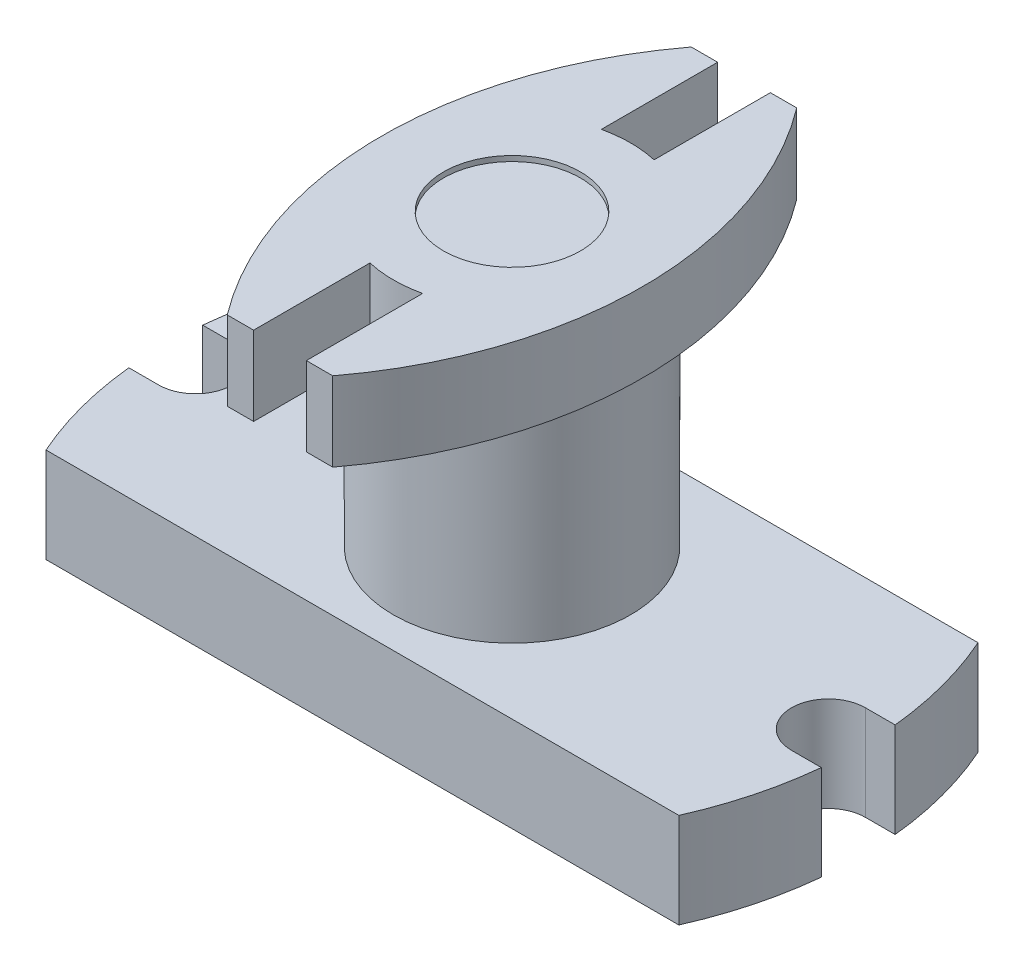
ISO-10303-21;
HEADER;
FILE_DESCRIPTION(('STEP AP214'),'2;1');
FILE_NAME('part.step','',(''),(''),'','','');
FILE_SCHEMA(('AUTOMOTIVE_DESIGN { 1 0 10303 214 1 1 1 1 }'));
ENDSEC;
DATA;
#1=APPLICATION_CONTEXT('core data for automotive mechanical design processes');
#2=APPLICATION_PROTOCOL_DEFINITION('international standard','automotive_design',2000,#1);
#3=PRODUCT_CONTEXT('',#1,'mechanical');
#4=PRODUCT('Part','Part','',(#3));
#5=PRODUCT_RELATED_PRODUCT_CATEGORY('part','',(#4));
#6=PRODUCT_DEFINITION_FORMATION('','',#4);
#7=PRODUCT_DEFINITION_CONTEXT('part definition',#1,'design');
#8=PRODUCT_DEFINITION('design','',#6,#7);
#9=PRODUCT_DEFINITION_SHAPE('','',#8);
#10=(LENGTH_UNIT() NAMED_UNIT(*) SI_UNIT(.MILLI.,.METRE.));
#11=(NAMED_UNIT(*) PLANE_ANGLE_UNIT() SI_UNIT($,.RADIAN.));
#12=(NAMED_UNIT(*) SI_UNIT($,.STERADIAN.) SOLID_ANGLE_UNIT());
#13=UNCERTAINTY_MEASURE_WITH_UNIT(LENGTH_MEASURE(1.E-05),#10,'distance_accuracy_value','');
#14=(GEOMETRIC_REPRESENTATION_CONTEXT(3) GLOBAL_UNCERTAINTY_ASSIGNED_CONTEXT((#13)) GLOBAL_UNIT_ASSIGNED_CONTEXT((#10,
#11,#12)) REPRESENTATION_CONTEXT('',''));
#15=CARTESIAN_POINT('',(0.,0.,0.));
#16=DIRECTION('',(0.,0.,1.));
#17=DIRECTION('',(1.,0.,0.));
#18=AXIS2_PLACEMENT_3D('',#15,#16,#17);
#19=CARTESIAN_POINT('',(-4.99999378583697,55.,0.));
#20=DIRECTION('',(1.,0.,0.));
#21=DIRECTION('',(0.,0.,-1.));
#22=AXIS2_PLACEMENT_3D('',#19,#20,#21);
#23=PLANE('',#22);
#24=DIRECTION('',(0.,0.,1.));
#25=VECTOR('',#24,1.);
#26=CARTESIAN_POINT('',(-4.99999378583697,40.,0.));
#27=LINE('',#26,#25);
#28=CARTESIAN_POINT('',(-4.99999378583697,40.,21.9374123848186));
#29=VERTEX_POINT('',#28);
#30=CARTESIAN_POINT('',(-4.99999378583697,40.,43.9921170061762));
#31=VERTEX_POINT('',#30);
#32=EDGE_CURVE('E221',#29,#31,#27,.T.);
#33=ORIENTED_EDGE('',*,*,#32,.F.);
#34=DIRECTION('',(0.,-1.,0.));
#35=VECTOR('',#34,1.);
#36=CARTESIAN_POINT('',(-4.99999378583697,55.,21.9374123848186));
#37=LINE('',#36,#35);
#38=CARTESIAN_POINT('',(-4.99999378583697,55.,21.9374123848186));
#39=VERTEX_POINT('',#38);
#40=EDGE_CURVE('E208',#39,#29,#37,.T.);
#41=ORIENTED_EDGE('',*,*,#40,.F.);
#42=DIRECTION('',(0.,0.,1.));
#43=VECTOR('',#42,1.);
#44=CARTESIAN_POINT('',(-4.99999378583697,55.,0.));
#45=LINE('',#44,#43);
#46=CARTESIAN_POINT('',(-4.99999378583697,55.,43.9921170061762));
#47=VERTEX_POINT('',#46);
#48=EDGE_CURVE('E218',#39,#47,#45,.T.);
#49=ORIENTED_EDGE('',*,*,#48,.T.);
#50=DIRECTION('',(0.,-1.,0.));
#51=VECTOR('',#50,1.);
#52=CARTESIAN_POINT('',(-4.99999378583697,55.,43.9921170061762));
#53=LINE('',#52,#51);
#54=EDGE_CURVE('E282',#47,#31,#53,.T.);
#55=ORIENTED_EDGE('',*,*,#54,.T.);
#56=EDGE_LOOP('',(#33,#41,#49,#55));
#57=FACE_BOUND('',#56,.T.);
#58=ADVANCED_FACE('F44',(#57),#23,.T.);
#59=CARTESIAN_POINT('',(4.99999378583698,55.,0.));
#60=DIRECTION('',(1.,0.,0.));
#61=DIRECTION('',(0.,0.,-1.));
#62=AXIS2_PLACEMENT_3D('',#59,#60,#61);
#63=PLANE('',#62);
#64=DIRECTION('',(0.,-1.,0.));
#65=VECTOR('',#64,1.);
#66=CARTESIAN_POINT('',(4.99999378583698,55.,21.9374123848186));
#67=LINE('',#66,#65);
#68=CARTESIAN_POINT('',(4.99999378583698,55.,21.9374123848186));
#69=VERTEX_POINT('',#68);
#70=CARTESIAN_POINT('',(4.99999378583698,40.,21.9374123848186));
#71=VERTEX_POINT('',#70);
#72=EDGE_CURVE('E65',#69,#71,#67,.T.);
#73=ORIENTED_EDGE('',*,*,#72,.T.);
#74=DIRECTION('',(0.,0.,1.));
#75=VECTOR('',#74,1.);
#76=CARTESIAN_POINT('',(4.99999378583698,40.,0.));
#77=LINE('',#76,#75);
#78=CARTESIAN_POINT('',(4.99999378583698,40.,43.9921170061762));
#79=VERTEX_POINT('',#78);
#80=EDGE_CURVE('E261',#71,#79,#77,.T.);
#81=ORIENTED_EDGE('',*,*,#80,.T.);
#82=DIRECTION('',(0.,-1.,0.));
#83=VECTOR('',#82,1.);
#84=CARTESIAN_POINT('',(4.99999378583698,55.,43.9921170061762));
#85=LINE('',#84,#83);
#86=CARTESIAN_POINT('',(4.99999378583698,55.,43.9921170061762));
#87=VERTEX_POINT('',#86);
#88=EDGE_CURVE('E279',#87,#79,#85,.T.);
#89=ORIENTED_EDGE('',*,*,#88,.F.);
#90=DIRECTION('',(0.,0.,1.));
#91=VECTOR('',#90,1.);
#92=CARTESIAN_POINT('',(4.99999378583698,55.,0.));
#93=LINE('',#92,#91);
#94=EDGE_CURVE('E230',#69,#87,#93,.T.);
#95=ORIENTED_EDGE('',*,*,#94,.F.);
#96=EDGE_LOOP('',(#73,#81,#89,#95));
#97=FACE_BOUND('',#96,.T.);
#98=ADVANCED_FACE('F442',(#97),#63,.F.);
#99=DIRECTION('',(0.,-1.,0.));
#100=VECTOR('',#99,1.);
#101=CARTESIAN_POINT('',(4.99999378583697,55.,-21.9374123848186));
#102=LINE('',#101,#100);
#103=CARTESIAN_POINT('',(4.99999378583698,55.,-21.9374123848186));
#104=VERTEX_POINT('',#103);
#105=CARTESIAN_POINT('',(4.99999378583698,40.,-21.9374123848186));
#106=VERTEX_POINT('',#105);
#107=EDGE_CURVE('E251',#104,#106,#102,.T.);
#108=ORIENTED_EDGE('',*,*,#107,.F.);
#109=CARTESIAN_POINT('',(4.99999378583698,55.,-43.9921170061762));
#110=VERTEX_POINT('',#109);
#111=EDGE_CURVE('E231',#110,#104,#93,.T.);
#112=ORIENTED_EDGE('',*,*,#111,.F.);
#113=DIRECTION('',(0.,-1.,0.));
#114=VECTOR('',#113,1.);
#115=CARTESIAN_POINT('',(4.99999378583698,55.,-43.9921170061762));
#116=LINE('',#115,#114);
#117=CARTESIAN_POINT('',(4.99999378583698,40.,-43.9921170061762));
#118=VERTEX_POINT('',#117);
#119=EDGE_CURVE('E240',#110,#118,#116,.T.);
#120=ORIENTED_EDGE('',*,*,#119,.T.);
#121=EDGE_CURVE('E265',#118,#106,#77,.T.);
#122=ORIENTED_EDGE('',*,*,#121,.T.);
#123=EDGE_LOOP('',(#108,#112,#120,#122));
#124=FACE_BOUND('',#123,.T.);
#125=ADVANCED_FACE('F448',(#124),#63,.F.);
#126=CARTESIAN_POINT('',(-4.99999378583697,55.,-43.9921170061762));
#127=VERTEX_POINT('',#126);
#128=CARTESIAN_POINT('',(-4.99999378583697,55.,-21.9374123848186));
#129=VERTEX_POINT('',#128);
#130=EDGE_CURVE('E70',#127,#129,#45,.T.);
#131=ORIENTED_EDGE('',*,*,#130,.T.);
#132=DIRECTION('',(0.,-1.,0.));
#133=VECTOR('',#132,1.);
#134=CARTESIAN_POINT('',(-4.99999378583697,55.,-21.9374123848186));
#135=LINE('',#134,#133);
#136=CARTESIAN_POINT('',(-4.99999378583697,40.,-21.9374123848186));
#137=VERTEX_POINT('',#136);
#138=EDGE_CURVE('E648',#129,#137,#135,.T.);
#139=ORIENTED_EDGE('',*,*,#138,.T.);
#140=CARTESIAN_POINT('',(-4.99999378583697,40.,-43.9921170061762));
#141=VERTEX_POINT('',#140);
#142=EDGE_CURVE('E262',#141,#137,#27,.T.);
#143=ORIENTED_EDGE('',*,*,#142,.F.);
#144=DIRECTION('',(0.,-1.,0.));
#145=VECTOR('',#144,1.);
#146=CARTESIAN_POINT('',(-4.99999378583697,55.,-43.9921170061762));
#147=LINE('',#146,#145);
#148=EDGE_CURVE('E236',#127,#141,#147,.T.);
#149=ORIENTED_EDGE('',*,*,#148,.F.);
#150=EDGE_LOOP('',(#131,#139,#143,#149));
#151=FACE_BOUND('',#150,.T.);
#152=ADVANCED_FACE('F444',(#151),#23,.T.);
#153=CARTESIAN_POINT('',(-3.99801441927227,-18.,0.));
#154=DIRECTION('',(0.,1.,0.));
#155=DIRECTION('',(0.,0.,1.));
#156=AXIS2_PLACEMENT_3D('',#153,#154,#155);
#157=CYLINDRICAL_SURFACE('',#156,70.);
#158=CARTESIAN_POINT('',(-3.99801441927227,0.,0.));
#159=DIRECTION('',(0.,1.,0.));
#160=DIRECTION('',(0.,0.,-1.));
#161=AXIS2_PLACEMENT_3D('',#158,#159,#160);
#162=CIRCLE('',#161,70.);
#163=CARTESIAN_POINT('',(60.,0.,28.359375));
#164=VERTEX_POINT('',#163);
#165=CARTESIAN_POINT('',(65.6511061781912,0.,6.99999999999999));
#166=VERTEX_POINT('',#165);
#167=EDGE_CURVE('E293',#164,#166,#162,.T.);
#168=ORIENTED_EDGE('',*,*,#167,.F.);
#169=DIRECTION('',(0.,1.,0.));
#170=VECTOR('',#169,1.);
#171=CARTESIAN_POINT('',(60.,-18.,28.359375));
#172=LINE('',#171,#170);
#173=CARTESIAN_POINT('',(60.,-18.,28.359375));
#174=VERTEX_POINT('',#173);
#175=EDGE_CURVE('E53',#174,#164,#172,.T.);
#176=ORIENTED_EDGE('',*,*,#175,.F.);
#177=CARTESIAN_POINT('',(-3.99801441927227,-18.,0.));
#178=DIRECTION('',(0.,1.,0.));
#179=DIRECTION('',(0.,0.,-1.));
#180=AXIS2_PLACEMENT_3D('',#177,#178,#179);
#181=CIRCLE('',#180,70.);
#182=CARTESIAN_POINT('',(65.6511061781912,-18.,6.99999999999999));
#183=VERTEX_POINT('',#182);
#184=EDGE_CURVE('E291',#174,#183,#181,.T.);
#185=ORIENTED_EDGE('',*,*,#184,.T.);
#186=DIRECTION('',(0.,1.,0.));
#187=VECTOR('',#186,1.);
#188=CARTESIAN_POINT('',(65.6511061781912,-18.,6.99999999999999));
#189=LINE('',#188,#187);
#190=EDGE_CURVE('E47',#183,#166,#189,.T.);
#191=ORIENTED_EDGE('',*,*,#190,.T.);
#192=EDGE_LOOP('',(#168,#176,#185,#191));
#193=FACE_BOUND('',#192,.T.);
#194=ADVANCED_FACE('F50',(#193),#157,.T.);
#195=CARTESIAN_POINT('',(-60.,-18.,28.359375));
#196=DIRECTION('',(0.,0.,1.));
#197=DIRECTION('',(1.,0.,0.));
#198=AXIS2_PLACEMENT_3D('',#195,#196,#197);
#199=PLANE('',#198);
#200=DIRECTION('',(1.,0.,0.));
#201=VECTOR('',#200,1.);
#202=CARTESIAN_POINT('',(-60.,0.,28.359375));
#203=LINE('',#202,#201);
#204=CARTESIAN_POINT('',(-60.,0.,28.359375));
#205=VERTEX_POINT('',#204);
#206=EDGE_CURVE('E300',#205,#164,#203,.T.);
#207=ORIENTED_EDGE('',*,*,#206,.F.);
#208=DIRECTION('',(0.,1.,0.));
#209=VECTOR('',#208,1.);
#210=CARTESIAN_POINT('',(-60.,-18.,28.359375));
#211=LINE('',#210,#209);
#212=CARTESIAN_POINT('',(-60.,-18.,28.359375));
#213=VERTEX_POINT('',#212);
#214=EDGE_CURVE('E362',#213,#205,#211,.T.);
#215=ORIENTED_EDGE('',*,*,#214,.F.);
#216=DIRECTION('',(1.,0.,0.));
#217=VECTOR('',#216,1.);
#218=CARTESIAN_POINT('',(-60.,-18.,28.359375));
#219=LINE('',#218,#217);
#220=EDGE_CURVE('E327',#213,#174,#219,.T.);
#221=ORIENTED_EDGE('',*,*,#220,.T.);
#222=ORIENTED_EDGE('',*,*,#175,.T.);
#223=EDGE_LOOP('',(#207,#215,#221,#222));
#224=FACE_BOUND('',#223,.T.);
#225=ADVANCED_FACE('F397',(#224),#199,.T.);
#226=CARTESIAN_POINT('',(3.99801441927227,-18.,0.));
#227=DIRECTION('',(0.,1.,0.));
#228=DIRECTION('',(0.,0.,1.));
#229=AXIS2_PLACEMENT_3D('',#226,#227,#228);
#230=CYLINDRICAL_SURFACE('',#229,70.);
#231=CARTESIAN_POINT('',(3.99801441927227,0.,0.));
#232=DIRECTION('',(0.,1.,0.));
#233=DIRECTION('',(0.,0.,1.));
#234=AXIS2_PLACEMENT_3D('',#231,#232,#233);
#235=CIRCLE('',#234,70.);
#236=CARTESIAN_POINT('',(-65.6511061781912,0.,6.99999999999999));
#237=VERTEX_POINT('',#236);
#238=EDGE_CURVE('E360',#237,#205,#235,.T.);
#239=ORIENTED_EDGE('',*,*,#238,.F.);
#240=DIRECTION('',(0.,1.,0.));
#241=VECTOR('',#240,1.);
#242=CARTESIAN_POINT('',(-65.6511061781912,-18.,6.99999999999999));
#243=LINE('',#242,#241);
#244=CARTESIAN_POINT('',(-65.6511061781912,-18.,6.99999999999999));
#245=VERTEX_POINT('',#244);
#246=EDGE_CURVE('E370',#245,#237,#243,.T.);
#247=ORIENTED_EDGE('',*,*,#246,.F.);
#248=CARTESIAN_POINT('',(3.99801441927227,-18.,0.));
#249=DIRECTION('',(0.,1.,0.));
#250=DIRECTION('',(0.,0.,1.));
#251=AXIS2_PLACEMENT_3D('',#248,#249,#250);
#252=CIRCLE('',#251,70.);
#253=EDGE_CURVE('E324',#245,#213,#252,.T.);
#254=ORIENTED_EDGE('',*,*,#253,.T.);
#255=ORIENTED_EDGE('',*,*,#214,.T.);
#256=EDGE_LOOP('',(#239,#247,#254,#255));
#257=FACE_BOUND('',#256,.T.);
#258=ADVANCED_FACE('F433',(#257),#230,.T.);
#259=CARTESIAN_POINT('',(-60.,-18.,6.99999999999999));
#260=DIRECTION('',(0.,0.,-1.));
#261=DIRECTION('',(-1.,0.,0.));
#262=AXIS2_PLACEMENT_3D('',#259,#260,#261);
#263=PLANE('',#262);
#264=DIRECTION('',(-1.,0.,0.));
#265=VECTOR('',#264,1.);
#266=CARTESIAN_POINT('',(-60.,0.,6.99999999999999));
#267=LINE('',#266,#265);
#268=CARTESIAN_POINT('',(-60.,0.,6.99999999999999));
#269=VERTEX_POINT('',#268);
#270=EDGE_CURVE('E358',#269,#237,#267,.T.);
#271=ORIENTED_EDGE('',*,*,#270,.F.);
#272=DIRECTION('',(0.,1.,0.));
#273=VECTOR('',#272,1.);
#274=CARTESIAN_POINT('',(-60.,-18.,6.99999999999999));
#275=LINE('',#274,#273);
#276=CARTESIAN_POINT('',(-60.,-18.,6.99999999999999));
#277=VERTEX_POINT('',#276);
#278=EDGE_CURVE('E367',#277,#269,#275,.T.);
#279=ORIENTED_EDGE('',*,*,#278,.F.);
#280=DIRECTION('',(-1.,0.,0.));
#281=VECTOR('',#280,1.);
#282=CARTESIAN_POINT('',(-60.,-18.,6.99999999999999));
#283=LINE('',#282,#281);
#284=EDGE_CURVE('E323',#277,#245,#283,.T.);
#285=ORIENTED_EDGE('',*,*,#284,.T.);
#286=ORIENTED_EDGE('',*,*,#246,.T.);
#287=EDGE_LOOP('',(#271,#279,#285,#286));
#288=FACE_BOUND('',#287,.T.);
#289=ADVANCED_FACE('F427',(#288),#263,.T.);
#290=CARTESIAN_POINT('',(-60.,-18.,0.));
#291=DIRECTION('',(0.,1.,0.));
#292=DIRECTION('',(0.,0.,1.));
#293=AXIS2_PLACEMENT_3D('',#290,#291,#292);
#294=CYLINDRICAL_SURFACE('',#293,6.99999999999998);
#295=CARTESIAN_POINT('',(-60.,0.,0.));
#296=DIRECTION('',(0.,-1.,0.));
#297=DIRECTION('',(0.,0.,1.));
#298=AXIS2_PLACEMENT_3D('',#295,#296,#297);
#299=CIRCLE('',#298,6.99999999999998);
#300=CARTESIAN_POINT('',(-60.,0.,-6.99999999999999));
#301=VERTEX_POINT('',#300);
#302=EDGE_CURVE('E354',#301,#269,#299,.T.);
#303=ORIENTED_EDGE('',*,*,#302,.F.);
#304=DIRECTION('',(0.,1.,0.));
#305=VECTOR('',#304,1.);
#306=CARTESIAN_POINT('',(-60.,-18.,-6.99999999999999));
#307=LINE('',#306,#305);
#308=CARTESIAN_POINT('',(-60.,-18.,-6.99999999999999));
#309=VERTEX_POINT('',#308);
#310=EDGE_CURVE('E371',#309,#301,#307,.T.);
#311=ORIENTED_EDGE('',*,*,#310,.F.);
#312=CARTESIAN_POINT('',(-60.,-18.,0.));
#313=DIRECTION('',(0.,-1.,0.));
#314=DIRECTION('',(0.,0.,1.));
#315=AXIS2_PLACEMENT_3D('',#312,#313,#314);
#316=CIRCLE('',#315,6.99999999999998);
#317=EDGE_CURVE('E319',#309,#277,#316,.T.);
#318=ORIENTED_EDGE('',*,*,#317,.T.);
#319=ORIENTED_EDGE('',*,*,#278,.T.);
#320=EDGE_LOOP('',(#303,#311,#318,#319));
#321=FACE_BOUND('',#320,.T.);
#322=ADVANCED_FACE('F430',(#321),#294,.F.);
#323=CARTESIAN_POINT('',(-60.,-18.,-6.99999999999998));
#324=DIRECTION('',(0.,0.,1.));
#325=DIRECTION('',(1.,0.,0.));
#326=AXIS2_PLACEMENT_3D('',#323,#324,#325);
#327=PLANE('',#326);
#328=DIRECTION('',(1.,0.,0.));
#329=VECTOR('',#328,1.);
#330=CARTESIAN_POINT('',(-60.,0.,-6.99999999999998));
#331=LINE('',#330,#329);
#332=CARTESIAN_POINT('',(-65.6511061781912,0.,-6.99999999999998));
#333=VERTEX_POINT('',#332);
#334=EDGE_CURVE('E350',#333,#301,#331,.T.);
#335=ORIENTED_EDGE('',*,*,#334,.F.);
#336=DIRECTION('',(0.,1.,0.));
#337=VECTOR('',#336,1.);
#338=CARTESIAN_POINT('',(-65.6511061781912,-18.,-6.99999999999998));
#339=LINE('',#338,#337);
#340=CARTESIAN_POINT('',(-65.6511061781912,-18.,-6.99999999999998));
#341=VERTEX_POINT('',#340);
#342=EDGE_CURVE('E373',#341,#333,#339,.T.);
#343=ORIENTED_EDGE('',*,*,#342,.F.);
#344=DIRECTION('',(1.,0.,0.));
#345=VECTOR('',#344,1.);
#346=CARTESIAN_POINT('',(-60.,-18.,-6.99999999999998));
#347=LINE('',#346,#345);
#348=EDGE_CURVE('E314',#341,#309,#347,.T.);
#349=ORIENTED_EDGE('',*,*,#348,.T.);
#350=ORIENTED_EDGE('',*,*,#310,.T.);
#351=EDGE_LOOP('',(#335,#343,#349,#350));
#352=FACE_BOUND('',#351,.T.);
#353=ADVANCED_FACE('F421',(#352),#327,.T.);
#354=CARTESIAN_POINT('',(3.99801441927227,-18.,0.));
#355=DIRECTION('',(0.,1.,0.));
#356=DIRECTION('',(0.,0.,1.));
#357=AXIS2_PLACEMENT_3D('',#354,#355,#356);
#358=CYLINDRICAL_SURFACE('',#357,70.);
#359=CARTESIAN_POINT('',(3.99801441927227,0.,0.));
#360=DIRECTION('',(0.,1.,0.));
#361=DIRECTION('',(0.,0.,1.));
#362=AXIS2_PLACEMENT_3D('',#359,#360,#361);
#363=CIRCLE('',#362,70.);
#364=CARTESIAN_POINT('',(-60.,0.,-28.359375));
#365=VERTEX_POINT('',#364);
#366=EDGE_CURVE('E347',#365,#333,#363,.T.);
#367=ORIENTED_EDGE('',*,*,#366,.F.);
#368=DIRECTION('',(0.,1.,0.));
#369=VECTOR('',#368,1.);
#370=CARTESIAN_POINT('',(-60.,-18.,-28.359375));
#371=LINE('',#370,#369);
#372=CARTESIAN_POINT('',(-60.,-18.,-28.359375));
#373=VERTEX_POINT('',#372);
#374=EDGE_CURVE('E374',#373,#365,#371,.T.);
#375=ORIENTED_EDGE('',*,*,#374,.F.);
#376=CARTESIAN_POINT('',(3.99801441927227,-18.,0.));
#377=DIRECTION('',(0.,1.,0.));
#378=DIRECTION('',(0.,0.,1.));
#379=AXIS2_PLACEMENT_3D('',#376,#377,#378);
#380=CIRCLE('',#379,70.);
#381=EDGE_CURVE('E315',#373,#341,#380,.T.);
#382=ORIENTED_EDGE('',*,*,#381,.T.);
#383=ORIENTED_EDGE('',*,*,#342,.T.);
#384=EDGE_LOOP('',(#367,#375,#382,#383));
#385=FACE_BOUND('',#384,.T.);
#386=ADVANCED_FACE('F418',(#385),#358,.T.);
#387=CARTESIAN_POINT('',(-60.,-18.,-28.359375));
#388=DIRECTION('',(0.,0.,-1.));
#389=DIRECTION('',(-1.,0.,0.));
#390=AXIS2_PLACEMENT_3D('',#387,#388,#389);
#391=PLANE('',#390);
#392=DIRECTION('',(-1.,0.,0.));
#393=VECTOR('',#392,1.);
#394=CARTESIAN_POINT('',(-60.,0.,-28.359375));
#395=LINE('',#394,#393);
#396=CARTESIAN_POINT('',(60.,0.,-28.359375));
#397=VERTEX_POINT('',#396);
#398=EDGE_CURVE('E344',#397,#365,#395,.T.);
#399=ORIENTED_EDGE('',*,*,#398,.F.);
#400=DIRECTION('',(0.,1.,0.));
#401=VECTOR('',#400,1.);
#402=CARTESIAN_POINT('',(60.,-18.,-28.359375));
#403=LINE('',#402,#401);
#404=CARTESIAN_POINT('',(60.,-18.,-28.359375));
#405=VERTEX_POINT('',#404);
#406=EDGE_CURVE('E380',#405,#397,#403,.T.);
#407=ORIENTED_EDGE('',*,*,#406,.F.);
#408=DIRECTION('',(-1.,0.,0.));
#409=VECTOR('',#408,1.);
#410=CARTESIAN_POINT('',(-60.,-18.,-28.359375));
#411=LINE('',#410,#409);
#412=EDGE_CURVE('E307',#405,#373,#411,.T.);
#413=ORIENTED_EDGE('',*,*,#412,.T.);
#414=ORIENTED_EDGE('',*,*,#374,.T.);
#415=EDGE_LOOP('',(#399,#407,#413,#414));
#416=FACE_BOUND('',#415,.T.);
#417=ADVANCED_FACE('F415',(#416),#391,.T.);
#418=CARTESIAN_POINT('',(-3.99801441927227,-18.,0.));
#419=DIRECTION('',(0.,1.,0.));
#420=DIRECTION('',(0.,0.,1.));
#421=AXIS2_PLACEMENT_3D('',#418,#419,#420);
#422=CYLINDRICAL_SURFACE('',#421,70.);
#423=CARTESIAN_POINT('',(-3.99801441927227,0.,0.));
#424=DIRECTION('',(0.,1.,0.));
#425=DIRECTION('',(0.,0.,-1.));
#426=AXIS2_PLACEMENT_3D('',#423,#424,#425);
#427=CIRCLE('',#426,70.);
#428=CARTESIAN_POINT('',(65.6511061781912,0.,-6.99999999999997));
#429=VERTEX_POINT('',#428);
#430=EDGE_CURVE('E343',#429,#397,#427,.T.);
#431=ORIENTED_EDGE('',*,*,#430,.F.);
#432=DIRECTION('',(0.,1.,0.));
#433=VECTOR('',#432,1.);
#434=CARTESIAN_POINT('',(65.6511061781912,-18.,-6.99999999999997));
#435=LINE('',#434,#433);
#436=CARTESIAN_POINT('',(65.6511061781912,-18.,-6.99999999999997));
#437=VERTEX_POINT('',#436);
#438=EDGE_CURVE('E378',#437,#429,#435,.T.);
#439=ORIENTED_EDGE('',*,*,#438,.F.);
#440=CARTESIAN_POINT('',(-3.99801441927227,-18.,0.));
#441=DIRECTION('',(0.,1.,0.));
#442=DIRECTION('',(0.,0.,-1.));
#443=AXIS2_PLACEMENT_3D('',#440,#441,#442);
#444=CIRCLE('',#443,70.);
#445=EDGE_CURVE('E306',#437,#405,#444,.T.);
#446=ORIENTED_EDGE('',*,*,#445,.T.);
#447=ORIENTED_EDGE('',*,*,#406,.T.);
#448=EDGE_LOOP('',(#431,#439,#446,#447));
#449=FACE_BOUND('',#448,.T.);
#450=ADVANCED_FACE('F411',(#449),#422,.T.);
#451=CARTESIAN_POINT('',(60.,-18.,-6.99999999999998));
#452=DIRECTION('',(0.,0.,1.));
#453=DIRECTION('',(1.,0.,0.));
#454=AXIS2_PLACEMENT_3D('',#451,#452,#453);
#455=PLANE('',#454);
#456=DIRECTION('',(1.,0.,0.));
#457=VECTOR('',#456,1.);
#458=CARTESIAN_POINT('',(60.,0.,-6.99999999999998));
#459=LINE('',#458,#457);
#460=CARTESIAN_POINT('',(60.,0.,-6.99999999999998));
#461=VERTEX_POINT('',#460);
#462=EDGE_CURVE('E336',#461,#429,#459,.T.);
#463=ORIENTED_EDGE('',*,*,#462,.F.);
#464=DIRECTION('',(0.,1.,0.));
#465=VECTOR('',#464,1.);
#466=CARTESIAN_POINT('',(60.,-18.,-6.99999999999998));
#467=LINE('',#466,#465);
#468=CARTESIAN_POINT('',(60.,-18.,-6.99999999999998));
#469=VERTEX_POINT('',#468);
#470=EDGE_CURVE('E382',#469,#461,#467,.T.);
#471=ORIENTED_EDGE('',*,*,#470,.F.);
#472=DIRECTION('',(1.,0.,0.));
#473=VECTOR('',#472,1.);
#474=CARTESIAN_POINT('',(60.,-18.,-6.99999999999998));
#475=LINE('',#474,#473);
#476=EDGE_CURVE('E303',#469,#437,#475,.T.);
#477=ORIENTED_EDGE('',*,*,#476,.T.);
#478=ORIENTED_EDGE('',*,*,#438,.T.);
#479=EDGE_LOOP('',(#463,#471,#477,#478));
#480=FACE_BOUND('',#479,.T.);
#481=ADVANCED_FACE('F409',(#480),#455,.T.);
#482=CARTESIAN_POINT('',(60.,-18.,0.));
#483=DIRECTION('',(0.,1.,0.));
#484=DIRECTION('',(0.,0.,1.));
#485=AXIS2_PLACEMENT_3D('',#482,#483,#484);
#486=CYLINDRICAL_SURFACE('',#485,6.99999999999998);
#487=CARTESIAN_POINT('',(60.,0.,0.));
#488=DIRECTION('',(0.,-1.,0.));
#489=DIRECTION('',(0.,0.,-1.));
#490=AXIS2_PLACEMENT_3D('',#487,#488,#489);
#491=CIRCLE('',#490,6.99999999999998);
#492=CARTESIAN_POINT('',(60.,0.,6.99999999999998));
#493=VERTEX_POINT('',#492);
#494=EDGE_CURVE('E333',#493,#461,#491,.T.);
#495=ORIENTED_EDGE('',*,*,#494,.F.);
#496=DIRECTION('',(0.,1.,0.));
#497=VECTOR('',#496,1.);
#498=CARTESIAN_POINT('',(60.,-18.,6.99999999999998));
#499=LINE('',#498,#497);
#500=CARTESIAN_POINT('',(60.,-18.,6.99999999999998));
#501=VERTEX_POINT('',#500);
#502=EDGE_CURVE('E385',#501,#493,#499,.T.);
#503=ORIENTED_EDGE('',*,*,#502,.F.);
#504=CARTESIAN_POINT('',(60.,-18.,0.));
#505=DIRECTION('',(0.,-1.,0.));
#506=DIRECTION('',(0.,0.,-1.));
#507=AXIS2_PLACEMENT_3D('',#504,#505,#506);
#508=CIRCLE('',#507,6.99999999999998);
#509=EDGE_CURVE('E297',#501,#469,#508,.T.);
#510=ORIENTED_EDGE('',*,*,#509,.T.);
#511=ORIENTED_EDGE('',*,*,#470,.T.);
#512=EDGE_LOOP('',(#495,#503,#510,#511));
#513=FACE_BOUND('',#512,.T.);
#514=ADVANCED_FACE('F403',(#513),#486,.F.);
#515=CARTESIAN_POINT('',(60.,-18.,6.99999999999999));
#516=DIRECTION('',(0.,0.,-1.));
#517=DIRECTION('',(-1.,0.,0.));
#518=AXIS2_PLACEMENT_3D('',#515,#516,#517);
#519=PLANE('',#518);
#520=DIRECTION('',(-1.,0.,0.));
#521=VECTOR('',#520,1.);
#522=CARTESIAN_POINT('',(60.,0.,6.99999999999999));
#523=LINE('',#522,#521);
#524=EDGE_CURVE('E334',#166,#493,#523,.T.);
#525=ORIENTED_EDGE('',*,*,#524,.F.);
#526=ORIENTED_EDGE('',*,*,#190,.F.);
#527=DIRECTION('',(-1.,0.,0.));
#528=VECTOR('',#527,1.);
#529=CARTESIAN_POINT('',(60.,-18.,6.99999999999999));
#530=LINE('',#529,#528);
#531=EDGE_CURVE('E298',#183,#501,#530,.T.);
#532=ORIENTED_EDGE('',*,*,#531,.T.);
#533=ORIENTED_EDGE('',*,*,#502,.T.);
#534=EDGE_LOOP('',(#525,#526,#532,#533));
#535=FACE_BOUND('',#534,.T.);
#536=ADVANCED_FACE('F387',(#535),#519,.T.);
#537=CARTESIAN_POINT('',(-3.99801441927227,-18.,0.));
#538=DIRECTION('',(0.,-1.,0.));
#539=DIRECTION('',(0.,0.,-1.));
#540=AXIS2_PLACEMENT_3D('',#537,#538,#539);
#541=PLANE('',#540);
#542=ORIENTED_EDGE('',*,*,#184,.F.);
#543=ORIENTED_EDGE('',*,*,#220,.F.);
#544=ORIENTED_EDGE('',*,*,#253,.F.);
#545=ORIENTED_EDGE('',*,*,#284,.F.);
#546=ORIENTED_EDGE('',*,*,#317,.F.);
#547=ORIENTED_EDGE('',*,*,#348,.F.);
#548=ORIENTED_EDGE('',*,*,#381,.F.);
#549=ORIENTED_EDGE('',*,*,#412,.F.);
#550=ORIENTED_EDGE('',*,*,#445,.F.);
#551=ORIENTED_EDGE('',*,*,#476,.F.);
#552=ORIENTED_EDGE('',*,*,#509,.F.);
#553=ORIENTED_EDGE('',*,*,#531,.F.);
#554=EDGE_LOOP('',(#542,#543,#544,#545,#546,#547,#548,#549,#550,#551,#552,#553));
#555=FACE_BOUND('',#554,.T.);
#556=ADVANCED_FACE('F396',(#555),#541,.T.);
#557=CARTESIAN_POINT('',(-3.99801441927227,0.,0.));
#558=DIRECTION('',(0.,-1.,0.));
#559=DIRECTION('',(0.,0.,-1.));
#560=AXIS2_PLACEMENT_3D('',#557,#558,#559);
#561=PLANE('',#560);
#562=CARTESIAN_POINT('',(0.,0.,0.));
#563=DIRECTION('',(0.,1.,0.));
#564=DIRECTION('',(0.,0.,1.));
#565=AXIS2_PLACEMENT_3D('',#562,#563,#564);
#566=CIRCLE('',#565,22.5);
#567=CARTESIAN_POINT('',(0.,0.,22.5));
#568=VERTEX_POINT('',#567);
#569=EDGE_CURVE('E11',#568,#568,#566,.T.);
#570=ORIENTED_EDGE('',*,*,#569,.F.);
#571=EDGE_LOOP('',(#570));
#572=FACE_BOUND('',#571,.T.);
#573=ORIENTED_EDGE('',*,*,#167,.T.);
#574=ORIENTED_EDGE('',*,*,#524,.T.);
#575=ORIENTED_EDGE('',*,*,#494,.T.);
#576=ORIENTED_EDGE('',*,*,#462,.T.);
#577=ORIENTED_EDGE('',*,*,#430,.T.);
#578=ORIENTED_EDGE('',*,*,#398,.T.);
#579=ORIENTED_EDGE('',*,*,#366,.T.);
#580=ORIENTED_EDGE('',*,*,#334,.T.);
#581=ORIENTED_EDGE('',*,*,#302,.T.);
#582=ORIENTED_EDGE('',*,*,#270,.T.);
#583=ORIENTED_EDGE('',*,*,#238,.T.);
#584=ORIENTED_EDGE('',*,*,#206,.T.);
#585=EDGE_LOOP('',(#573,#574,#575,#576,#577,#578,#579,#580,#581,#582,#583,#584));
#586=FACE_BOUND('',#585,.T.);
#587=ADVANCED_FACE('F392',(#572,#586),#561,.F.);
#588=CARTESIAN_POINT('',(0.,40.,0.));
#589=DIRECTION('',(0.,-1.,0.));
#590=DIRECTION('',(0.,0.,-1.));
#591=AXIS2_PLACEMENT_3D('',#588,#589,#590);
#592=CYLINDRICAL_SURFACE('',#591,22.5);
#593=CARTESIAN_POINT('',(0.,40.,0.));
#594=DIRECTION('',(0.,1.,0.));
#595=DIRECTION('',(0.,0.,1.));
#596=AXIS2_PLACEMENT_3D('',#593,#594,#595);
#597=CIRCLE('',#596,22.5);
#598=EDGE_CURVE('E290',#71,#106,#597,.T.);
#599=ORIENTED_EDGE('',*,*,#598,.F.);
#600=ORIENTED_EDGE('',*,*,#72,.F.);
#601=CARTESIAN_POINT('',(0.,55.,-3.12250225675825E-13));
#602=DIRECTION('',(0.,1.,0.));
#603=DIRECTION('',(0.,0.,1.));
#604=AXIS2_PLACEMENT_3D('',#601,#602,#603);
#605=CIRCLE('',#604,22.5000000000003);
#606=EDGE_CURVE('E203',#39,#69,#605,.T.);
#607=ORIENTED_EDGE('',*,*,#606,.F.);
#608=ORIENTED_EDGE('',*,*,#40,.T.);
#609=EDGE_CURVE('E288',#137,#29,#597,.T.);
#610=ORIENTED_EDGE('',*,*,#609,.F.);
#611=ORIENTED_EDGE('',*,*,#138,.F.);
#612=CARTESIAN_POINT('',(0.,55.,0.));
#613=DIRECTION('',(0.,1.,0.));
#614=DIRECTION('',(0.,0.,-1.));
#615=AXIS2_PLACEMENT_3D('',#612,#613,#614);
#616=CIRCLE('',#615,22.5);
#617=EDGE_CURVE('E224',#104,#129,#616,.T.);
#618=ORIENTED_EDGE('',*,*,#617,.F.);
#619=ORIENTED_EDGE('',*,*,#107,.T.);
#620=EDGE_LOOP('',(#599,#600,#607,#608,#610,#611,#618,#619));
#621=FACE_BOUND('',#620,.T.);
#622=ORIENTED_EDGE('',*,*,#569,.T.);
#623=EDGE_LOOP('',(#622));
#624=FACE_BOUND('',#623,.T.);
#625=ADVANCED_FACE('F210',(#621,#624),#592,.T.);
#626=CARTESIAN_POINT('',(0.,40.,0.));
#627=DIRECTION('',(0.,1.,0.));
#628=DIRECTION('',(0.,0.,1.));
#629=AXIS2_PLACEMENT_3D('',#626,#627,#628);
#630=PLANE('',#629);
#631=ORIENTED_EDGE('',*,*,#80,.F.);
#632=ORIENTED_EDGE('',*,*,#598,.T.);
#633=ORIENTED_EDGE('',*,*,#121,.F.);
#634=DIRECTION('',(1.,0.,0.));
#635=VECTOR('',#634,1.);
#636=CARTESIAN_POINT('',(0.,40.,-43.9921170061762));
#637=LINE('',#636,#635);
#638=CARTESIAN_POINT('',(9.99999378583697,40.,-43.9921170061762));
#639=VERTEX_POINT('',#638);
#640=EDGE_CURVE('E268',#118,#639,#637,.T.);
#641=ORIENTED_EDGE('',*,*,#640,.T.);
#642=CARTESIAN_POINT('',(-48.2554234842754,40.,0.));
#643=DIRECTION('',(0.,1.,0.));
#644=DIRECTION('',(0.,0.,1.));
#645=AXIS2_PLACEMENT_3D('',#642,#643,#644);
#646=CIRCLE('',#645,73.);
#647=CARTESIAN_POINT('',(9.99999378583698,40.,43.9921170061762));
#648=VERTEX_POINT('',#647);
#649=EDGE_CURVE('E269',#648,#639,#646,.T.);
#650=ORIENTED_EDGE('',*,*,#649,.F.);
#651=DIRECTION('',(1.,0.,0.));
#652=VECTOR('',#651,1.);
#653=CARTESIAN_POINT('',(0.,40.,43.9921170061762));
#654=LINE('',#653,#652);
#655=EDGE_CURVE('E263',#79,#648,#654,.T.);
#656=ORIENTED_EDGE('',*,*,#655,.F.);
#657=EDGE_LOOP('',(#631,#632,#633,#641,#650,#656));
#658=FACE_BOUND('',#657,.T.);
#659=ADVANCED_FACE('F490',(#658),#630,.F.);
#660=ORIENTED_EDGE('',*,*,#142,.T.);
#661=ORIENTED_EDGE('',*,*,#609,.T.);
#662=ORIENTED_EDGE('',*,*,#32,.T.);
#663=DIRECTION('',(-1.,0.,0.));
#664=VECTOR('',#663,1.);
#665=CARTESIAN_POINT('',(0.,40.,43.9921170061762));
#666=LINE('',#665,#664);
#667=CARTESIAN_POINT('',(-9.99999378583697,40.,43.9921170061762));
#668=VERTEX_POINT('',#667);
#669=EDGE_CURVE('E260',#31,#668,#666,.T.);
#670=ORIENTED_EDGE('',*,*,#669,.T.);
#671=CARTESIAN_POINT('',(48.2554234842753,40.,0.));
#672=DIRECTION('',(0.,1.,0.));
#673=DIRECTION('',(0.,0.,1.));
#674=AXIS2_PLACEMENT_3D('',#671,#672,#673);
#675=CIRCLE('',#674,73.);
#676=CARTESIAN_POINT('',(-9.99999378583698,40.,-43.9921170061762));
#677=VERTEX_POINT('',#676);
#678=EDGE_CURVE('E254',#677,#668,#675,.T.);
#679=ORIENTED_EDGE('',*,*,#678,.F.);
#680=DIRECTION('',(-1.,0.,0.));
#681=VECTOR('',#680,1.);
#682=CARTESIAN_POINT('',(0.,40.,-43.9921170061762));
#683=LINE('',#682,#681);
#684=EDGE_CURVE('E249',#141,#677,#683,.T.);
#685=ORIENTED_EDGE('',*,*,#684,.F.);
#686=EDGE_LOOP('',(#660,#661,#662,#670,#679,#685));
#687=FACE_BOUND('',#686,.T.);
#688=ADVANCED_FACE('F488',(#687),#630,.F.);
#689=CARTESIAN_POINT('',(0.,55.,-43.9921170061762));
#690=DIRECTION('',(0.,0.,1.));
#691=DIRECTION('',(1.,0.,0.));
#692=AXIS2_PLACEMENT_3D('',#689,#690,#691);
#693=PLANE('',#692);
#694=ORIENTED_EDGE('',*,*,#684,.T.);
#695=DIRECTION('',(0.,-1.,0.));
#696=VECTOR('',#695,1.);
#697=CARTESIAN_POINT('',(-9.99999378583698,55.,-43.9921170061762));
#698=LINE('',#697,#696);
#699=CARTESIAN_POINT('',(-9.99999378583698,55.,-43.9921170061762));
#700=VERTEX_POINT('',#699);
#701=EDGE_CURVE('E286',#700,#677,#698,.T.);
#702=ORIENTED_EDGE('',*,*,#701,.F.);
#703=DIRECTION('',(-1.,0.,0.));
#704=VECTOR('',#703,1.);
#705=CARTESIAN_POINT('',(0.,55.,-43.9921170061762));
#706=LINE('',#705,#704);
#707=EDGE_CURVE('E647',#127,#700,#706,.T.);
#708=ORIENTED_EDGE('',*,*,#707,.F.);
#709=ORIENTED_EDGE('',*,*,#148,.T.);
#710=EDGE_LOOP('',(#694,#702,#708,#709));
#711=FACE_BOUND('',#710,.T.);
#712=ADVANCED_FACE('F482',(#711),#693,.F.);
#713=CARTESIAN_POINT('',(48.2554234842753,55.,0.));
#714=DIRECTION('',(0.,-1.,0.));
#715=DIRECTION('',(0.,0.,-1.));
#716=AXIS2_PLACEMENT_3D('',#713,#714,#715);
#717=CYLINDRICAL_SURFACE('',#716,73.);
#718=ORIENTED_EDGE('',*,*,#678,.T.);
#719=DIRECTION('',(0.,-1.,0.));
#720=VECTOR('',#719,1.);
#721=CARTESIAN_POINT('',(-9.99999378583697,55.,43.9921170061762));
#722=LINE('',#721,#720);
#723=CARTESIAN_POINT('',(-9.99999378583697,55.,43.9921170061762));
#724=VERTEX_POINT('',#723);
#725=EDGE_CURVE('E283',#724,#668,#722,.T.);
#726=ORIENTED_EDGE('',*,*,#725,.F.);
#727=CARTESIAN_POINT('',(48.2554234842753,55.,0.));
#728=DIRECTION('',(0.,1.,0.));
#729=DIRECTION('',(0.,0.,1.));
#730=AXIS2_PLACEMENT_3D('',#727,#728,#729);
#731=CIRCLE('',#730,73.);
#732=EDGE_CURVE('E234',#700,#724,#731,.T.);
#733=ORIENTED_EDGE('',*,*,#732,.F.);
#734=ORIENTED_EDGE('',*,*,#701,.T.);
#735=EDGE_LOOP('',(#718,#726,#733,#734));
#736=FACE_BOUND('',#735,.T.);
#737=ADVANCED_FACE('F479',(#736),#717,.T.);
#738=CARTESIAN_POINT('',(0.,55.,43.9921170061762));
#739=DIRECTION('',(0.,0.,1.));
#740=DIRECTION('',(1.,0.,0.));
#741=AXIS2_PLACEMENT_3D('',#738,#739,#740);
#742=PLANE('',#741);
#743=ORIENTED_EDGE('',*,*,#669,.F.);
#744=ORIENTED_EDGE('',*,*,#54,.F.);
#745=DIRECTION('',(-1.,0.,0.));
#746=VECTOR('',#745,1.);
#747=CARTESIAN_POINT('',(0.,55.,43.9921170061762));
#748=LINE('',#747,#746);
#749=EDGE_CURVE('E226',#47,#724,#748,.T.);
#750=ORIENTED_EDGE('',*,*,#749,.T.);
#751=ORIENTED_EDGE('',*,*,#725,.T.);
#752=EDGE_LOOP('',(#743,#744,#750,#751));
#753=FACE_BOUND('',#752,.T.);
#754=ADVANCED_FACE('F474',(#753),#742,.T.);
#755=CARTESIAN_POINT('',(0.,55.,43.9921170061762));
#756=DIRECTION('',(0.,0.,-1.));
#757=DIRECTION('',(-1.,0.,0.));
#758=AXIS2_PLACEMENT_3D('',#755,#756,#757);
#759=PLANE('',#758);
#760=ORIENTED_EDGE('',*,*,#655,.T.);
#761=DIRECTION('',(0.,-1.,0.));
#762=VECTOR('',#761,1.);
#763=CARTESIAN_POINT('',(9.99999378583698,55.,43.9921170061762));
#764=LINE('',#763,#762);
#765=CARTESIAN_POINT('',(9.99999378583698,55.,43.9921170061762));
#766=VERTEX_POINT('',#765);
#767=EDGE_CURVE('E278',#766,#648,#764,.T.);
#768=ORIENTED_EDGE('',*,*,#767,.F.);
#769=DIRECTION('',(1.,0.,0.));
#770=VECTOR('',#769,1.);
#771=CARTESIAN_POINT('',(0.,55.,43.9921170061762));
#772=LINE('',#771,#770);
#773=EDGE_CURVE('E233',#87,#766,#772,.T.);
#774=ORIENTED_EDGE('',*,*,#773,.F.);
#775=ORIENTED_EDGE('',*,*,#88,.T.);
#776=EDGE_LOOP('',(#760,#768,#774,#775));
#777=FACE_BOUND('',#776,.T.);
#778=ADVANCED_FACE('F468',(#777),#759,.F.);
#779=CARTESIAN_POINT('',(-48.2554234842754,55.,0.));
#780=DIRECTION('',(0.,-1.,0.));
#781=DIRECTION('',(0.,0.,-1.));
#782=AXIS2_PLACEMENT_3D('',#779,#780,#781);
#783=CYLINDRICAL_SURFACE('',#782,73.);
#784=ORIENTED_EDGE('',*,*,#649,.T.);
#785=DIRECTION('',(0.,-1.,0.));
#786=VECTOR('',#785,1.);
#787=CARTESIAN_POINT('',(9.99999378583697,55.,-43.9921170061762));
#788=LINE('',#787,#786);
#789=CARTESIAN_POINT('',(9.99999378583697,55.,-43.9921170061762));
#790=VERTEX_POINT('',#789);
#791=EDGE_CURVE('E274',#790,#639,#788,.T.);
#792=ORIENTED_EDGE('',*,*,#791,.F.);
#793=CARTESIAN_POINT('',(-48.2554234842754,55.,0.));
#794=DIRECTION('',(0.,1.,0.));
#795=DIRECTION('',(0.,0.,1.));
#796=AXIS2_PLACEMENT_3D('',#793,#794,#795);
#797=CIRCLE('',#796,73.);
#798=EDGE_CURVE('E244',#766,#790,#797,.T.);
#799=ORIENTED_EDGE('',*,*,#798,.F.);
#800=ORIENTED_EDGE('',*,*,#767,.T.);
#801=EDGE_LOOP('',(#784,#792,#799,#800));
#802=FACE_BOUND('',#801,.T.);
#803=ADVANCED_FACE('F467',(#802),#783,.T.);
#804=CARTESIAN_POINT('',(0.,55.,-43.9921170061762));
#805=DIRECTION('',(0.,0.,-1.));
#806=DIRECTION('',(-1.,0.,0.));
#807=AXIS2_PLACEMENT_3D('',#804,#805,#806);
#808=PLANE('',#807);
#809=ORIENTED_EDGE('',*,*,#640,.F.);
#810=ORIENTED_EDGE('',*,*,#119,.F.);
#811=DIRECTION('',(1.,0.,0.));
#812=VECTOR('',#811,1.);
#813=CARTESIAN_POINT('',(0.,55.,-43.9921170061762));
#814=LINE('',#813,#812);
#815=EDGE_CURVE('E239',#110,#790,#814,.T.);
#816=ORIENTED_EDGE('',*,*,#815,.T.);
#817=ORIENTED_EDGE('',*,*,#791,.T.);
#818=EDGE_LOOP('',(#809,#810,#816,#817));
#819=FACE_BOUND('',#818,.T.);
#820=ADVANCED_FACE('F461',(#819),#808,.T.);
#821=CARTESIAN_POINT('',(0.,55.,0.));
#822=DIRECTION('',(0.,1.,0.));
#823=DIRECTION('',(0.,0.,1.));
#824=AXIS2_PLACEMENT_3D('',#821,#822,#823);
#825=PLANE('',#824);
#826=CARTESIAN_POINT('',(0.,55.,0.));
#827=DIRECTION('',(0.,1.,0.));
#828=DIRECTION('',(0.,0.,1.));
#829=AXIS2_PLACEMENT_3D('',#826,#827,#828);
#830=CIRCLE('',#829,12.9914924949852);
#831=CARTESIAN_POINT('',(0.,55.,12.9914924949852));
#832=VERTEX_POINT('',#831);
#833=EDGE_CURVE('E638',#832,#832,#830,.T.);
#834=ORIENTED_EDGE('',*,*,#833,.F.);
#835=EDGE_LOOP('',(#834));
#836=FACE_BOUND('',#835,.T.);
#837=ORIENTED_EDGE('',*,*,#48,.F.);
#838=ORIENTED_EDGE('',*,*,#606,.T.);
#839=ORIENTED_EDGE('',*,*,#94,.T.);
#840=ORIENTED_EDGE('',*,*,#773,.T.);
#841=ORIENTED_EDGE('',*,*,#798,.T.);
#842=ORIENTED_EDGE('',*,*,#815,.F.);
#843=ORIENTED_EDGE('',*,*,#111,.T.);
#844=ORIENTED_EDGE('',*,*,#617,.T.);
#845=ORIENTED_EDGE('',*,*,#130,.F.);
#846=ORIENTED_EDGE('',*,*,#707,.T.);
#847=ORIENTED_EDGE('',*,*,#732,.T.);
#848=ORIENTED_EDGE('',*,*,#749,.F.);
#849=EDGE_LOOP('',(#837,#838,#839,#840,#841,#842,#843,#844,#845,#846,#847,#848));
#850=FACE_BOUND('',#849,.T.);
#851=ADVANCED_FACE('F228',(#836,#850),#825,.T.);
#852=CARTESIAN_POINT('',(0.,54.,0.));
#853=DIRECTION('',(0.,1.,0.));
#854=DIRECTION('',(0.,0.,1.));
#855=AXIS2_PLACEMENT_3D('',#852,#853,#854);
#856=CYLINDRICAL_SURFACE('',#855,12.9914924949852);
#857=CARTESIAN_POINT('',(0.,54.,0.));
#858=DIRECTION('',(0.,1.,0.));
#859=DIRECTION('',(0.,0.,1.));
#860=AXIS2_PLACEMENT_3D('',#857,#858,#859);
#861=CIRCLE('',#860,12.9914924949852);
#862=CARTESIAN_POINT('',(0.,54.,12.9914924949852));
#863=VERTEX_POINT('',#862);
#864=EDGE_CURVE('E212',#863,#863,#861,.T.);
#865=ORIENTED_EDGE('',*,*,#864,.F.);
#866=EDGE_LOOP('',(#865));
#867=FACE_BOUND('',#866,.T.);
#868=ORIENTED_EDGE('',*,*,#833,.T.);
#869=EDGE_LOOP('',(#868));
#870=FACE_BOUND('',#869,.T.);
#871=ADVANCED_FACE('F542',(#867,#870),#856,.F.);
#872=CARTESIAN_POINT('',(0.,54.,0.));
#873=DIRECTION('',(0.,1.,0.));
#874=DIRECTION('',(0.,0.,1.));
#875=AXIS2_PLACEMENT_3D('',#872,#873,#874);
#876=PLANE('',#875);
#877=ORIENTED_EDGE('',*,*,#864,.T.);
#878=EDGE_LOOP('',(#877));
#879=FACE_BOUND('',#878,.T.);
#880=ADVANCED_FACE('F621',(#879),#876,.T.);
#881=CLOSED_SHELL('',(#58,#98,#125,#152,#194,#225,#258,#289,#322,#353,#386,#417,#450,#481,#514,
#536,#556,#587,#625,#659,#688,#712,#737,#754,#778,#803,#820,#851,#871,#880));
#882=MANIFOLD_SOLID_BREP('B2',#881);
#883=ADVANCED_BREP_SHAPE_REPRESENTATION('',(#18,#882),#14);
#884=SHAPE_DEFINITION_REPRESENTATION(#9,#883);
ENDSEC;
END-ISO-10303-21;
